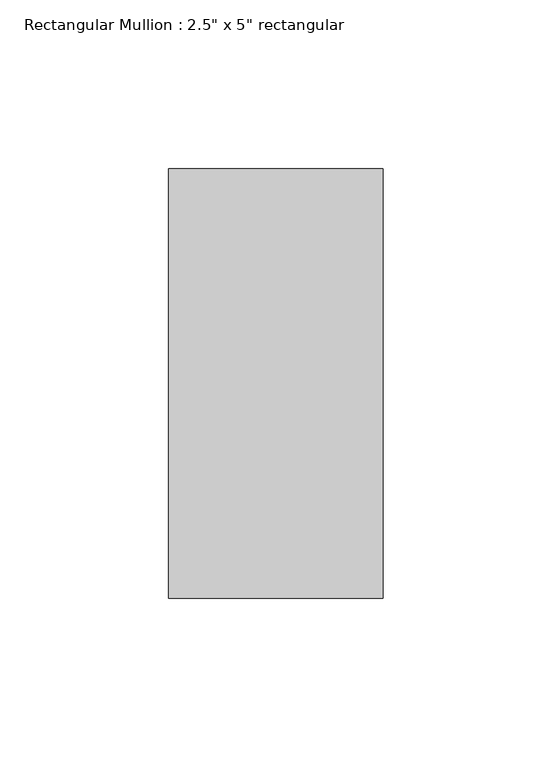
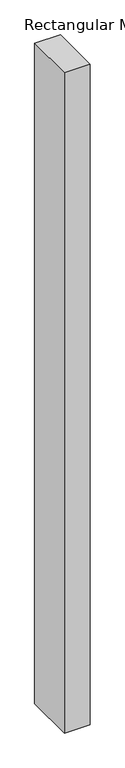
"""IFC4 building model written with IfcOpenShell, lengths in millimetres: member geometry."""

from ifc_helpers import new_model, si_unit, frame, origin, place, context, project, spatial, polyline, outline, extrude, source, transform, mapped, element, save


def member_427039da(model_context):
    return source(origin(), model_context, "Body", "SweptSolid", [
        extrude(outline(polyline([(0.0, 63.5), (0.0, -63.5), (-63.5, -63.5), (-63.5, 63.5), (0.0, 63.5)])), frame((0.0, 0.0, -1720.7849865), z_axis=(0.0, 0.0, 1.0), x_axis=(1.0, 0.0, 0.0)), (0.0, 0.0, 1.0), 1720.7849865),
    ])


if __name__ == "__main__":
    model = new_model("IFC4")
    model_context = context("Model", 3, world=origin())
    ifc_project = project(units=[si_unit("LENGTHUNIT", "METRE", prefix="MILLI")], contexts=[model_context])
    site = spatial("IfcSite", under=ifc_project)
    building = spatial("IfcBuilding", under=site)
    placement = place(None, origin())
    member_shape = member_427039da(model_context)
    element("IfcMember", 1, ObjectType="Rectangular Mullion : 2.5\" x 5\" rectangular", at=placement, inside=building, context=model_context, shape_type="MappedRepresentation", body=[
        mapped(member_shape, transform((0.0, 0.0, 0.0), x_axis=(1.0, 0.0, 0.0), y_axis=(0.0, 1.0, 0.0), z_axis=(0.0, 0.0, 1.0))),
    ])
    save(model, "model.ifc")

# Revit data of these elements
# Type "Rectangular Mullion : 2.5\" x 5\" rectangular"
#   built-in parameter 1007304 = 0.416667 (stored number, unit not read)
#   built-in parameter 1007301 = 0.104167 (stored number, unit not read)
#   built-in parameter 1007300 = 0.104167 (stored number, unit not read)
# Element 1 (IfcMember, "Rectangular Mullion : 2.5\" x 5\" rectangular")
#   Materials on its faces: "Aluminum"
# Materials
#   "Aluminum": class "Metal", colour RGB 247 247 247, transparency 0, Description = "Aluminum 6061", Cost = 0
